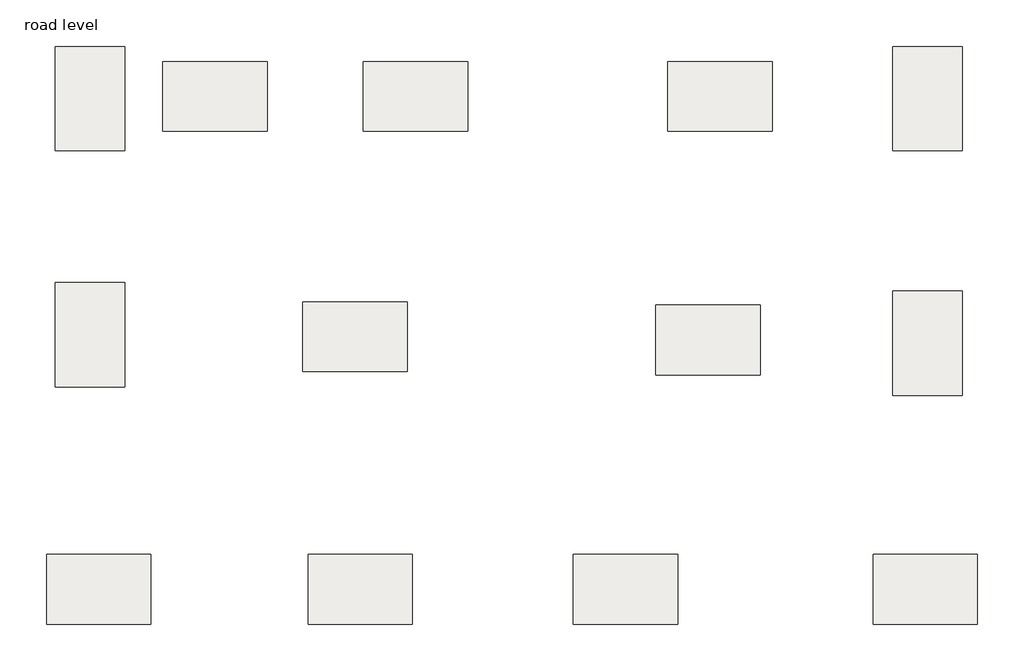
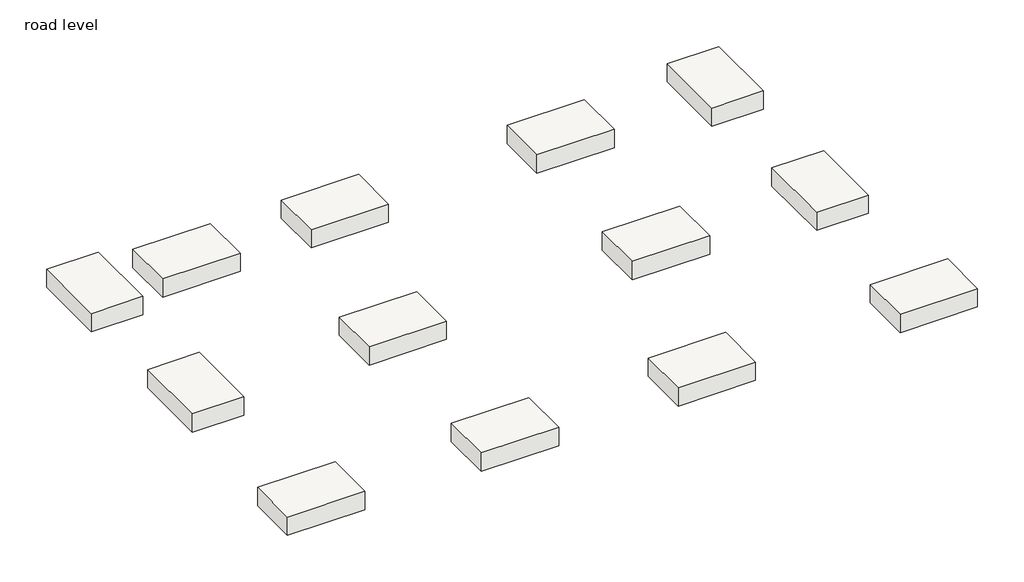
# One storey: 13 slabs.
"""IFC4 building model written with IfcOpenShell, lengths in millimetres."""

from ifc_helpers import new_model, si_unit, origin, place, context, project, spatial, transform, mapped, element, save
from components import slab_5ba74754

model = new_model("IFC4")

# Units and contexts
model_context = context("Model", 3, world=origin())
ifc_project = project(units=[si_unit("LENGTHUNIT", "METRE", prefix="MILLI")], contexts=[model_context])

# Site, building, storey
site = spatial("IfcSite", under=ifc_project)
building = spatial("IfcBuilding", under=site)
storey = spatial("IfcBuildingStorey", under=building, Name="road level", Elevation=0.0)

# Slabs
placement = place(None, origin())
slab_shape = slab_5ba74754(model_context)
element("IfcSlab", 1, ObjectType="Footing-Rectangular : 72\" x 48\" x 18\"", at=placement, inside=storey, context=model_context, shape_type="MappedRepresentation", body=[
    mapped(slab_shape, transform((-12757.668339, 9396.693496, -1219.2), x_axis=(1.0, 0.0, 0.0), y_axis=(0.0, 1.0, 0.0), z_axis=(0.0, 0.0, 1.0))),
])
element("IfcSlab", 2, ObjectType="Footing-Rectangular : 72\" x 48\" x 18\"", at=placement, inside=storey, context=model_context, shape_type="MappedRepresentation", body=[
    mapped(slab_shape, transform((-10566.918339, 9434.793496, -1219.2), x_axis=(0.0, 1.0, 0.0), y_axis=(-1.0, 0.0, 0.0), z_axis=(0.0, 0.0, 1.0))),
])
element("IfcSlab", 3, ObjectType="Footing-Rectangular : 72\" x 48\" x 18\"", at=placement, inside=storey, context=model_context, shape_type="MappedRepresentation", body=[
    mapped(slab_shape, transform((-7061.718339, 9434.793496, -1219.2), x_axis=(0.0, 1.0, 0.0), y_axis=(-1.0, 0.0, 0.0), z_axis=(0.0, 0.0, 1.0))),
])
element("IfcSlab", 4, ObjectType="Footing-Rectangular : 72\" x 48\" x 18\"", at=placement, inside=storey, context=model_context, shape_type="MappedRepresentation", body=[
    mapped(slab_shape, transform((-1727.718339, 9434.793496, -1219.2), x_axis=(0.0, 1.0, 0.0), y_axis=(-1.0, 0.0, 0.0), z_axis=(0.0, 0.0, 1.0))),
])
element("IfcSlab", 5, ObjectType="Footing-Rectangular : 72\" x 48\" x 18\"", at=placement, inside=storey, context=model_context, shape_type="MappedRepresentation", body=[
    mapped(slab_shape, transform((1904.481661, 9396.693496, -1219.2), x_axis=(-1.0, 0.0, 0.0), y_axis=(0.0, -1.0, 0.0), z_axis=(0.0, 0.0, 1.0))),
])
element("IfcSlab", 6, ObjectType="Footing-Rectangular : 72\" x 48\" x 18\"", at=placement, inside=storey, context=model_context, shape_type="MappedRepresentation", body=[
    mapped(slab_shape, transform((1904.481661, 5110.443496, -1219.2), x_axis=(-1.0, 0.0, 0.0), y_axis=(0.0, -1.0, 0.0), z_axis=(0.0, 0.0, 1.0))),
])
element("IfcSlab", 7, ObjectType="Footing-Rectangular : 72\" x 48\" x 18\"", at=placement, inside=storey, context=model_context, shape_type="MappedRepresentation", body=[
    mapped(slab_shape, transform((-1937.268339, 5167.593496, -1219.2), x_axis=(0.0, -1.0, 0.0), y_axis=(1.0, 0.0, 0.0), z_axis=(0.0, 0.0, 1.0))),
])
element("IfcSlab", 8, ObjectType="Footing-Rectangular : 72\" x 48\" x 18\"", at=placement, inside=storey, context=model_context, shape_type="MappedRepresentation", body=[
    mapped(slab_shape, transform((-8122.168339, 5224.743496, -1219.2), x_axis=(0.0, -1.0, 0.0), y_axis=(1.0, 0.0, 0.0), z_axis=(0.0, 0.0, 1.0))),
])
element("IfcSlab", 9, ObjectType="Footing-Rectangular : 72\" x 48\" x 18\"", at=placement, inside=storey, context=model_context, shape_type="MappedRepresentation", body=[
    mapped(slab_shape, transform((-12757.668339, 5262.843496, -1219.2), x_axis=(1.0, 0.0, 0.0), y_axis=(0.0, 1.0, 0.0), z_axis=(0.0, 0.0, 1.0))),
])
element("IfcSlab", 10, ObjectType="Footing-Rectangular : 72\" x 48\" x 18\"", at=placement, inside=storey, context=model_context, shape_type="MappedRepresentation", body=[
    mapped(slab_shape, transform((-12605.268339, 798.793496, -1219.2), x_axis=(0.0, 1.0, 0.0), y_axis=(-1.0, 0.0, 0.0), z_axis=(0.0, 0.0, 1.0))),
])
element("IfcSlab", 11, ObjectType="Footing-Rectangular : 72\" x 48\" x 18\"", at=placement, inside=storey, context=model_context, shape_type="MappedRepresentation", body=[
    mapped(slab_shape, transform((-8026.918339, 798.793496, -1219.2), x_axis=(0.0, 1.0, 0.0), y_axis=(-1.0, 0.0, 0.0), z_axis=(0.0, 0.0, 1.0))),
])
element("IfcSlab", 12, ObjectType="Footing-Rectangular : 72\" x 48\" x 18\"", at=placement, inside=storey, context=model_context, shape_type="MappedRepresentation", body=[
    mapped(slab_shape, transform((-3378.616739, 798.793496, -1219.2), x_axis=(0.0, 1.0, 0.0), y_axis=(-1.0, 0.0, 0.0), z_axis=(0.0, 0.0, 1.0))),
])
element("IfcSlab", 13, ObjectType="Footing-Rectangular : 72\" x 48\" x 18\"", at=placement, inside=storey, context=model_context, shape_type="MappedRepresentation", body=[
    mapped(slab_shape, transform((1866.381661, 798.793496, -1219.2), x_axis=(0.0, 1.0, 0.0), y_axis=(-1.0, 0.0, 0.0), z_axis=(0.0, 0.0, 1.0))),
])

save(model, "model.ifc")

# Revit data of these elements
# Type "Footing-Rectangular : 72\" x 48\" x 18\""
#   Assembly Code = "A1010100"
#   Width = 4 ft
#   Length = 6 ft
#   Foundation Thickness = 1.5 ft
#   Structural Material [instance default] = Concrete, Cast-in-Place gray
# Elements 1, 2, 3, 4, 5, 6, 7, 8, 9, 10, 11, 12, 13 (IfcSlab, "Footing-Rectangular : 72\" x 48\" x 18\"")
#   Structural Material = Concrete, Cast-in-Place gray
#   Phase Created = New Construction
#   Materials on its faces: "Concrete, Cast-in-Place gray"
# Materials
#   "Concrete, Cast-in-Place gray": class "Concrete", colour RGB 192 192 192, transparency 0, Description = "Cast-in-place concrete", Cost = 0
